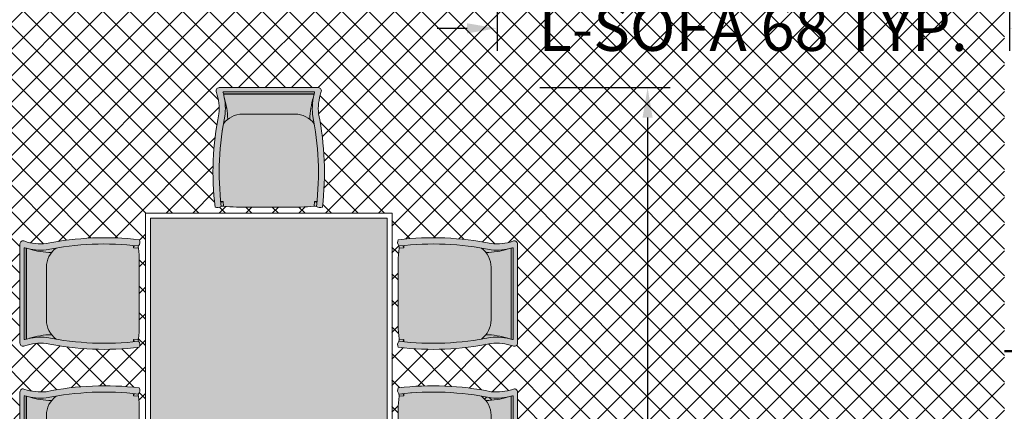
# Model space of a CAD drawing. Units: inches. Extents: x -466983 to 1020, y 324 to 318697.
# Tile 85 of 97: x 679 to 810, y 827 to 879. Entities that reach past the tile are written whole.
import ezdxf

# ---------------------------------------------------------------- set-up
doc = ezdxf.new("R2010")
doc.units = ezdxf.units.IN
doc.header["$MEASUREMENT"] = 0
for name, color, linetype, lineweight in [('A-ANNO-DIMS', 2, 'Continuous', 18), ('A-FLOR-PATT', 252, 'Continuous', 13), ('A-FURN', 8, 'Continuous', 18), ('A-WALL', 7, 'Continuous', 50)]:
    doc.layers.add(name, color=color, linetype=linetype, lineweight=lineweight)
doc.styles.get("Standard").update_dxf_attribs({"font": 'arial.ttf'})
doc.dimstyles.get("Standard").update_dxf_attribs({"dimtxt": 6, "dimasz": 4, "dimexe": 3, "dimexo": 3, "dimgap": 0.09, "dimtad": 0, "dimtih": 1, "dimtoh": 1, "dimdec": 1, "dimzin": 0, "dimdsep": 46, "dimlunit": 3, "dimtxsty": 'Standard', "dimcen": 0.09, "dimadec": 0, "dimazin": 0, "dimtfac": 1, "dimtdec": 1, "dimtofl": 0, "dimtmove": 0, "dimatfit": 3, "dimfxl": 1, "dimtolj": 1, "dimtzin": 0, "dimarcsym": 0})

# ---------------------------------------------------------------- blocks, each defined once
blk = doc.blocks.new('A$C51F1')
h = blk.add_hatch(color=256)
h.dxf.hatch_style = 1
h.paths.add_polyline_path([(0.4279, 0.4929), (0.026, 0.4929, 0.585109), (0.0153, 0.4737, -0.102523), (0.0249, 0.3863, 0.080461), (0.0093, 0.0091, 0.3023), (0.0338, 0.012, -0.012942), (0.0343, 0.0123, -0.080591), (0.05, 0.3835, 0.086627), (0.0435, 0.4661, -0.308377), (0.0433, 0.4665, -0.237278), (0.0433, 0.4671, 0.005839), (0.0418, 0.4726, -0.471786), (0.0436, 0.4758), (0.2273, 0.4758), (0.4111, 0.4758, -0.471786), (0.4129, 0.4726, 0.005839), (0.4114, 0.4671, -0.293853), (0.4112, 0.4664, 0.08699), (0.4047, 0.3835, -0.080655), (0.4203, 0.012, 0.301773), (0.4447, 0.0091, 0.080461), (0.4291, 0.3863, -0.102523), (0.4387, 0.4737, 0.587111)])
h.paths.add_polyline_path([(0.4107, 0.4676), (0.2273, 0.4676), (0.0439, 0.4676, 0.311255), (0.0433, 0.4671, -0.000568), (0.0434, 0.4666, -0.365297), (0.0439, 0.4668), (0.2273, 0.4668), (0.4107, 0.4668, -0.365297), (0.4113, 0.4666, -0.000568), (0.4114, 0.4671, 0.311255)], flags=17)
h = blk.add_hatch(color=256)
h.dxf.hatch_style = 1
h.paths.add_polyline_path([(0.4117, 0.3464, 0.23459), (0.3341, 0.3858), (0.2273, 0.3858), (0.1205, 0.3858, 0.165743), (0.061, 0.3649, 0.071703), (0.0463, 0.4542, -0.071168), (0.0502, 0.3861, 0.080361), (0.0343, 0.0123, -0.184513), (0.0429, 0.0127, 0.028193), (0.097, 0.0091), (0.227, 0.0091), (0.3571, 0.0091, 0.028193), (0.4111, 0.0127, -0.198751), (0.4203, 0.012, 0.072468)])
h.paths.add_polyline_path([(0.4084, 0.4542, -0.01323), (0.4113, 0.4666, 0.365297), (0.4107, 0.4668, 0.310553), (0.4107, 0.4676), (0.0439, 0.4676, 0.311255), (0.0433, 0.4671, -0.013798), (0.0463, 0.4542, -0.071703), (0.061, 0.3649, -0.165743), (0.1205, 0.3858), (0.2273, 0.3858), (0.3341, 0.3858, -0.165743), (0.3937, 0.3649, -0.071703)])
h.paths.add_polyline_path([(0.4047, 0.3835, -0.073923), (0.4084, 0.4542, 0.071703), (0.3937, 0.3649, -0.06627), (0.4117, 0.3464, 0.008137)], flags=17)
h.paths.add_polyline_path([(0.413, 0.473, 0.415817), (0.4111, 0.4758), (0.0436, 0.4758, 0.415817), (0.0416, 0.473, -0.006308), (0.0433, 0.4671, -0.311255), (0.0439, 0.4676), (0.4107, 0.4676, -0.336555), (0.4114, 0.4671, -0.006308)])
h = blk.add_hatch(color=256)
h.dxf.hatch_style = 1
h.paths.add_polyline_path([(0.4084, 0.4542, -0.01323), (0.4113, 0.4666, 0.365297), (0.4107, 0.4668), (0.2273, 0.4668), (0.0436, 0.4668, 0.193526), (0.0434, 0.4666, -0.01323), (0.0463, 0.4542, -0.071703), (0.061, 0.3649, -0.165743), (0.1205, 0.3858), (0.2273, 0.3858), (0.3341, 0.3858, -0.165743), (0.3937, 0.3649, -0.071703)])
at = {"color": 0}
for p, q in [((0.0436, 0.4758), (0.4111, 0.4758)), ((0.0439, 0.4676), (0.4107, 0.4676)), ((0.2273, 0.4668), (0.0439, 0.4668)), ((0.2273, 0.4668), (0.4107, 0.4668)), ((0.2273, 0.3858), (0.1205, 0.3858)), ((0.2273, 0.3858), (0.3341, 0.3858)), ((0.0417, 0.0321), (0.0321, 0.0321)), ((0.0417, 0.0321), (0.0326, 0.0278)), ((0.0435, 0.0127), (0.0417, 0.0321)), ((0.4112, 0.0127), (0.4129, 0.0321)), ((0.4129, 0.0321), (0.4225, 0.0321)), ((0.4129, 0.0321), (0.4221, 0.0278))]:
    blk.add_line(p, q, dxfattribs=at)
blk.add_lwpolyline([(0.4387, 0.4737, 0.102523), (0.4291, 0.3863, -0.080461), (0.4447, 0.0091, -0.3023), (0.4203, 0.012, 0.197932), (0.4111, 0.0127, -0.028193), (0.3571, 0.0091), (0.227, 0.0091), (0.097, 0.0091, -0.028193), (0.0429, 0.0127, 0.197932), (0.0338, 0.012, -0.3023), (0.0093, 0.0091, -0.080461), (0.0249, 0.3863, 0.102523), (0.0153, 0.4737, -0.587111), (0.0261, 0.4929), (0.4279, 0.4929, -0.587111)], format="xyb", close=True, dxfattribs=at)
for centre, radius, start, end in [((0.044, 0.4735), 0.00242, 100.345, 201.3742), ((-0.1898, 0.4063), 0.2409, 355.1793, 16.07), ((0.0439, 0.4669), 0.000725, 87.3762, 197.5208), ((0.0438, 0.4664), 0.000433, 71.7715, 189.2202), ((-0.2563, 0.3584), 0.3173, 1.1591, 17.5641), ((0.7109, 0.3584), 0.3173, 162.4359, 178.8409), ((0.6445, 0.4063), 0.2409, 164.0374, 185.4487), ((0.4107, 0.4669), 0.000725, 342.4792, 92.6238), ((0.4109, 0.4664), 0.000433, 350.7798, 108.2285), ((0.4106, 0.4735), 0.00242, 338.6258, 79.655), ((1.1976, 0.1501), 1.1714, 168.378, 186.769), ((0.1214, 0.2879), 0.0978, 90.5164, 143.1927), ((0.3332, 0.2879), 0.0978, 36.8073, 89.4836), ((-0.7314, 0.1497), 1.1599, 353.1854, 11.6291), ((0.0397, 0.0013), 0.012, 71.7536, 116.5375), ((0.4149, 0.0013), 0.012, 63.4625, 108.2464)]:
    blk.add_arc(centre, radius, start, end, dxfattribs=at)
blk = doc.blocks.new('Dining Table 1')
h = blk.add_hatch(color=256)
h.dxf.hatch_style = 1
h.set_gradient(color1=(0, 107, 0), color2=(254, 234, 185), name='INVSPHERICAL')
h.paths.add_polyline_path([(1939.98, 1142.68), (1908.44, 1142.68), (1908.44, 1061.84), (1939.98, 1061.84)])
at = {"ltscale": 0.5}
for points in [[(1907.78, 1143.33), (1907.78, 1061.19), (1940.64, 1061.19), (1940.64, 1143.33)], [(1908.44, 1142.68), (1908.44, 1061.84), (1939.98, 1061.84), (1939.98, 1142.68)]]:
    blk.add_lwpolyline(points, close=True, dxfattribs=at)
at = {"ltscale": 0.5, "xscale": 32.85880592291654, "yscale": 32.85880592291654, "zscale": 32.85880592291654}
blk.add_blockref('A$C51F1', (1916.75, 1143.86), dxfattribs=at)
at = {"ltscale": 0.5, "yscale": 32.85880592291654, "zscale": 32.85880592291654}
for p, xscale, rotation in [((1907.26, 1140.11), -32.85880592291654, 90), ((1941.16, 1140.11), 32.85880592291654, 270), ((1907.26, 1120.4), -32.85880592291654, 90), ((1941.16, 1120.4), 32.85880592291654, 270), ((1907.26, 1085.76), 32.85880592291654, 89.99999999999999), ((1941.16, 1085.76), -32.85880592291654, 270), ((1907.26, 1064.41), 32.85880592291654, 89.99999999999999), ((1941.16, 1064.41), -32.85880592291654, 270), ((1916.75, 1060.66), -32.85880592291654, 180)]:
    blk.add_blockref('A$C51F1', p, dxfattribs=dict(at, xscale=xscale, rotation=rotation))
blk = doc.blocks.new('*D71')
at = {"layer": 'A-ANNO-DIMS', "color": 0, "lineweight": -2, "transparency": 16777216}
for p, q in [((742.22, 885.15), (742.22, 874.91)), ((810.49, 885.15), (810.49, 874.91)), ((738.22, 877.91), (734.22, 877.91)), ((814.49, 877.91), (818.49, 877.91))]:
    blk.add_line(p, q, dxfattribs=at)
at = {"layer": 'A-ANNO-DIMS', "color": 0, "transparency": 16777216}
for points in [[(738.22, 878.58), (738.22, 877.24), (742.22, 877.91)], [(814.49, 878.58), (814.49, 877.24), (810.49, 877.91)]]:
    blk.add_solid(points, dxfattribs=at)
at = {"layer": 'Defpoints', "color": 0, "transparency": 16777216}
for p in [(742.22, 888.15), (810.49, 888.15), (742.22, 877.91)]:
    blk.add_point(p, dxfattribs=at)
at = {"layer": 'A-ANNO-DIMS', "color": 0, "transparency": 16777216, "insert": (776.35, 877.91), "char_height": 6, "attachment_point": 5}
blk.add_mtext('\\A1;L-SOFA 68 TYP.', dxfattribs=at)
blk = doc.blocks.new('*D111')
at = {"layer": 'A-ANNO-DIMS', "color": 0, "lineweight": -2, "transparency": 16777216}
for p, q in [((747.94, 870.02), (765.28, 870.02)), ((762.28, 866.02), (762.28, 815.42)), ((762.28, 758.43), (762.28, 809.03)), ((747.94, 754.43), (765.28, 754.43))]:
    blk.add_line(p, q, dxfattribs=at)
at = {"layer": 'A-ANNO-DIMS', "color": 0, "transparency": 16777216}
for points in [[(761.61, 866.02), (762.95, 866.02), (762.28, 870.02)], [(761.61, 758.43), (762.95, 758.43), (762.28, 754.43)]]:
    blk.add_solid(points, dxfattribs=at)
at = {"layer": 'Defpoints', "color": 0, "transparency": 16777216}
for p in [(744.94, 870.02), (762.28, 870.02), (744.94, 754.43)]:
    blk.add_point(p, dxfattribs=at)
at = {"layer": 'A-ANNO-DIMS', "color": 0, "transparency": 16777216, "insert": (762.28, 812.23), "char_height": 6, "attachment_point": 5}
blk.add_mtext('\\A1;DINING SET 116', dxfattribs=at)

msp = doc.modelspace()

# ---------------------------------------------------------------- hatches: boundary and pattern name
at = {"layer": 'A-FLOR-PATT', "transparency": 33554572}
h = msp.add_hatch(dxfattribs=at)
h.set_pattern_fill('ANSI37', color=256, scale=30)
h.set_pattern_definition([(45, (-1212.4137, -290.035), (-2.6516504, 2.6516504), []), (135, (-1212.4137, -290.035), (-2.6516504, -2.6516504), [])])
h.paths.add_polyline_path([(901.81, 1075.94), (900.61, 1075.94), (900.61, 1065.39), (899.39, 1065.39), (898.09, 1065.39), (892.84, 1058.71, -0.258377), (892.19, 1058.35), (879.98, 1058.35, -0.20177), (879.44, 1058.58), (874.08, 1065.39), (872.78, 1065.39), (871.56, 1065.39), (871.56, 1075.94), (813.81, 1075.94), (813.81, 1044.79), (832.39, 1044.79, -0.394795), (848.66, 1028.54), (848.66, 1009.94), (901.81, 1009.94), (901.81, 1015.94), (901.31, 1015.94), (871.31, 1015.94), (871.31, 1017.25), (871.33, 1017.25, -0.401453), (901.31, 1045.94), (901.81, 1045.94)])
edge = h.paths.add_edge_path(flags=16)
edge.add_line((847.77, 1068.95), (847.77, 1073.71))
edge.add_arc((849.23, 1073.71), 1.45, 90, 180, ccw=False)
edge.add_line((849.23, 1075.16), (864.49, 1075.16))
edge.add_arc((864.49, 1073.71), 1.45, 0, 90, ccw=False)
edge.add_line((865.95, 1073.71), (865.95, 1069))
edge.add_arc((832.64, 1068.98), 33.3, -20.6123, 0.0472, ccw=False)
edge.add_ellipse((856.86, 1058.48), major_axis=(0, 10.21), ratio=0.685919, start_angle=100.0088, end_angle=259.9912, ccw=False)
edge.add_arc((881.07, 1068.98), 33.3, 180.0472, 200.6123, ccw=False)
h.paths.add_polyline_path([(853.15, 1066.48), (853.15, 1066.45), (853.15, 1066.45, 0.433107), (852.92, 1066.68), (852.92, 1066.45), (853.15, 1066.45), (853.15, 1066.48), (853.09, 1066.61, 0.697939), (852.7, 1066.45), (852.7, 1066.45), (852.7, 1066.48), (852.92, 1067), (852.92, 1066.68, -0.396254)], flags=0)
h.paths.add_polyline_path([(861.02, 1066.48), (861.02, 1066.45), (861.02, 1066.45, 0.416404), (860.8, 1066.68), (860.8, 1066.45), (861.02, 1066.45), (861.02, 1066.48), (860.97, 1066.61, 0.713344), (860.57, 1066.45), (860.57, 1066.45), (860.57, 1066.48), (860.8, 1067), (860.8, 1066.68, -0.379973)], flags=0)
edge = h.paths.add_edge_path(flags=0)
edge.add_spline(control_points=[(861.13, 1065.79), (861.47, 1065.25), (861.61, 1065.02), (861.98, 1064.37), (862.19, 1063.94), (862.56, 1063.04), (862.72, 1062.56), (862.99, 1061.58), (863.09, 1061.07), (863.25, 1060.03), (863.29, 1059.5), (863.33, 1058.44), (863.32, 1057.91), (863.24, 1056.85), (863.17, 1056.33), (862.97, 1055.31), (862.84, 1054.81), (862.54, 1053.85), (862.36, 1053.39), (861.95, 1052.52), (861.73, 1052.12), (861.23, 1051.36), (860.97, 1051.02), (860.4, 1050.39), (860.11, 1050.12), (859.49, 1049.65), (859.18, 1049.45), (858.53, 1049.13), (858.2, 1049.01), (857.53, 1048.85), (857.2, 1048.81), (856.52, 1048.81), (856.19, 1048.85), (855.52, 1049.01), (855.19, 1049.13), (854.54, 1049.45), (854.23, 1049.64), (853.61, 1050.12), (853.32, 1050.39), (852.75, 1051.01), (852.49, 1051.36), (852, 1052.11), (851.77, 1052.52), (851.36, 1053.39), (851.18, 1053.85), (850.88, 1054.81), (850.75, 1055.31), (850.55, 1056.33), (850.48, 1056.85), (850.4, 1057.9), (850.39, 1058.44), (850.43, 1059.5), (850.47, 1060.03), (850.63, 1061.07), (850.73, 1061.58), (851, 1062.56), (851.16, 1063.04), (851.53, 1063.94), (851.73, 1064.37), (852.11, 1065.02), (852.25, 1065.25), (852.61, 1065.73)], knot_values=[3.915332, 3.915332, 3.915332, 3.915332, 4.013468, 4.013468, 4.175532, 4.175532, 4.337596, 4.337596, 4.49966, 4.49966, 4.661724, 4.661724, 4.823788, 4.823788, 4.985852, 4.985852, 5.147916, 5.147916, 5.30998, 5.30998, 5.472044, 5.472044, 5.634109, 5.634109, 5.796173, 5.796173, 5.958237, 5.958237, 6.120301, 6.120301, 6.282365, 6.282365, 6.444429, 6.444429, 6.606493, 6.606493, 6.768557, 6.768557, 6.930621, 6.930621, 7.092685, 7.092685, 7.254749, 7.254749, 7.416813, 7.416813, 7.578878, 7.578878, 7.740942, 7.740942, 7.903006, 7.903006, 8.06507, 8.06507, 8.227134, 8.227134, 8.389198, 8.389198, 8.551262, 8.551262, 8.65037, 8.65037, 8.65037, 8.65037], degree=3, periodic=0)
edge.add_line((852.64, 1065.79), (861.13, 1065.79))
edge = h.paths.add_edge_path(flags=0)
edge.add_ellipse((856.85, 1057.74), major_axis=(0, 7.79), ratio=0.687861, start_angle=0, end_angle=360)
h.paths.add_polyline_path([(848.86, 1069.39), (848.86, 1073.96, -0.414214), (849.95, 1075.05), (863.77, 1075.05, -0.414214), (864.86, 1073.96), (864.86, 1069.39, -0.388936), (864.52, 1069.03, -0.043561), (849.2, 1069.03, -0.388936)], flags=0)
h.paths.add_polyline_path([(853.1, 1068.11, -1), (852.68, 1068.11, -1)], flags=0)
edge = h.paths.add_edge_path(flags=0)
edge.add_ellipse((856.86, 1057.34), major_axis=(0, 2.21), ratio=0.657164, start_angle=0, end_angle=360)
h.paths.add_polyline_path([(861.04, 1068.11, -1), (860.62, 1068.11, -1)], flags=0)
edge = h.paths.add_edge_path()
edge.add_line((573.95, 1057.34), (573.95, 1075.94))
edge.add_line((573.95, 1075.94), (558.73, 1075.94))
edge.add_line((558.73, 1075.94), (558.73, 1065.39))
edge.add_line((558.73, 1065.39), (557.51, 1065.39))
edge.add_line((557.51, 1065.39), (556.21, 1065.39))
edge.add_line((556.21, 1065.39), (550.95, 1058.71))
edge.add_arc((550.3, 1059.12), 0.765, 270, 327.9483, ccw=False)
edge.add_line((550.3, 1058.35), (538.1, 1058.35))
edge.add_arc((538.1, 1059.12), 0.765, 224.3704, 270, ccw=False)
edge.add_line((537.55, 1058.58), (532.2, 1065.39))
edge.add_line((532.2, 1065.39), (530.9, 1065.39))
edge.add_line((530.9, 1065.39), (529.67, 1065.39))
edge.add_line((529.67, 1065.39), (529.67, 1075.94))
edge.add_line((529.67, 1075.94), (520.81, 1075.94))
edge.add_line((520.81, 1075.94), (520.81, 1045.94))
edge.add_line((520.81, 1045.94), (521.31, 1045.94))
edge.add_arc((521.31, 1015.94), 30, 2.5075, 90, ccw=False)
edge.add_line((551.28, 1017.25), (551.31, 1017.25))
edge.add_line((551.31, 1017.25), (551.31, 1015.94))
edge.add_line((551.31, 1015.94), (520.81, 1015.94))
edge.add_line((520.81, 1015.94), (520.81, 1009.94))
edge.add_line((520.81, 1009.94), (559.19, 1010.4))
edge.add_arc((559.19, 1011.86), 1.45, 180, 270, ccw=False)
edge.add_line((557.74, 1011.86), (557.74, 1016.56))
edge.add_arc((591.04, 1016.59), 33.3, 159.3877, 180.0472, ccw=False)
edge.add_ellipse((566.82, 1027.08), major_axis=(0, 10.21), ratio=0.685919, start_angle=280.0088, end_angle=439.9912, ccw=False)
edge.add_arc((542.61, 1016.59), 33.3, 0.0472, 20.6123, ccw=False)
edge.add_line((575.91, 1016.62), (575.91, 1011.86))
edge.add_arc((574.46, 1011.86), 1.45, -90, 0, ccw=False)
edge.add_line((574.46, 1010.4), (608.81, 1009.94))
edge.add_line((608.81, 1009.94), (608.81, 1041.09))
edge.add_line((608.81, 1041.09), (590.22, 1041.09))
edge.add_arc((590.78, 1057.91), 16.83, 181.9277, 268.1032, ccw=False)
edge = h.paths.add_edge_path()
edge.add_ellipse((494.24, 583.62), major_axis=(0, 10.21), ratio=0.685919, start_angle=280.0088, end_angle=439.9912, ccw=False)
edge.add_arc((470.03, 573.12), 33.3, 0.0472, 20.6123, ccw=False)
edge.add_line((503.33, 573.15), (503.33, 568.39))
edge.add_arc((501.88, 568.39), 1.45, -90, 0, ccw=False)
edge.add_line((501.88, 566.94), (539.81, 566.94))
edge.add_line((539.81, 566.94), (539.81, 572.94))
edge.add_line((539.81, 572.94), (539.31, 572.94))
edge.add_line((539.31, 572.94), (509.31, 572.94))
edge.add_line((509.31, 572.94), (509.31, 574.25))
edge.add_line((509.31, 574.25), (509.33, 574.25))
edge.add_arc((539.31, 572.94), 30, 90, 177.4925, ccw=False)
edge.add_line((539.31, 602.94), (539.81, 602.94))
edge.add_line((539.81, 602.94), (539.81, 626.94))
edge.add_line((539.81, 626.94), (531.77, 626.94))
edge.add_line((531.77, 626.94), (531.77, 616.39))
edge.add_line((531.77, 616.39), (530.55, 616.39))
edge.add_line((530.55, 616.39), (529.25, 616.39))
edge.add_line((529.25, 616.39), (523.71, 609.35))
edge.add_line((523.71, 609.35), (510.78, 609.35))
edge.add_line((510.78, 609.35), (505.24, 616.39))
edge.add_line((505.24, 616.39), (503.94, 616.39))
edge.add_line((503.94, 616.39), (502.72, 616.39))
edge.add_line((502.72, 616.39), (502.72, 626.94))
edge.add_line((502.72, 626.94), (481.7, 626.94))
edge.add_line((481.7, 626.94), (481.7, 611))
edge.add_arc((467.27, 611.47), 14.44, 271.9277, 358.1032, ccw=False)
edge.add_line((467.76, 597.05), (451.81, 597.05))
edge.add_line((451.81, 597.05), (451.81, 584.4))
edge.add_line((451.81, 584.4), (451.81, 566.94))
edge.add_line((451.81, 566.94), (486.61, 566.94))
edge.add_arc((486.61, 568.39), 1.45, 180, 270, ccw=False)
edge.add_line((485.16, 568.39), (485.16, 573.1))
edge.add_arc((518.46, 573.12), 33.3, 159.3877, 180.0472, ccw=False)
h.paths.add_polyline_path([(836.26, 1020.73), (879.89, 1020.73), (879.89, 1039.39), (836.26, 1039.39)], flags=25)
h.paths.add_polyline_path([(549.99, 1036.75), (593.61, 1036.75), (593.61, 1055.41), (549.99, 1055.41)], flags=24)
h.paths.add_polyline_path([(475.12, 595.6), (518.75, 595.6), (518.75, 614.25), (475.12, 614.25)], flags=24)
h = msp.add_hatch(dxfattribs=at)
h.set_pattern_fill('ANSI37', color=256, scale=20)
h.set_pattern_definition([(45, (-1212.4137, -290.035), (-1.767767, 1.767767), []), (135, (-1212.4137, -290.035), (-1.767767, -1.767767), [])])
h.paths.add_polyline_path([(809.81, 870.94), (809.81, 888.15), (807, 888.15), (802.66, 888.15), (789.38, 888.15), (786.28, 888.15, -0.414214), (785.5, 888.94), (785.5, 900.2), (785.5, 908.47, -0.414214), (786.81, 909.78, -0.414214), (785.5, 911.09), (785.5, 929.1, -0.414214), (786.81, 930.41, -0.414214), (785.5, 931.72), (785.5, 931.9, -0.414214), (784.19, 930.59), (766.72, 930.59, -0.412359), (765.41, 931.9, -0.413741), (764.11, 930.58), (744.58, 930.42, -0.416556), (743.79, 931.21), (743.79, 933.52), (742.22, 933.52), (742.22, 952.02, -0.001344), (743.79, 952.2), (743.79, 953.94), (678.59, 953.94), (678.59, 951.13), (678.59, 946.79), (678.59, 933.52), (678.59, 930.42, -0.414214), (677.81, 929.63), (666.55, 929.63), (658.27, 929.63, -0.414214), (656.96, 930.94, -0.414214), (655.66, 929.63), (637.64, 929.63, -0.414214), (636.33, 930.94, -0.414214), (635.02, 929.63), (634.84, 929.63, -0.414214), (636.15, 928.32), (636.15, 910.85, -0.412359), (634.85, 909.55, -0.413741), (636.17, 908.25), (636.32, 888.71, -0.416556), (635.54, 887.92), (633.23, 887.92), (633.23, 886.35), (614.72, 886.35, -0.001344), (614.54, 887.92), (612.81, 887.92), (612.81, 834.94), (612.81, 752.94), (612.81, 748.94), (612.81, 697.94), (654.81, 697.94), (654.81, 701.94), (715.81, 701.94), (715.81, 737.44), (774.29, 737.44), (774.29, 795.94), (809.81, 795.94)])
h.paths.add_polyline_path([(679.28, 849.58, 0.102523), (682.15, 849.26, -0.080461), (694.54, 849.77, -0.283899), (694.48, 849.01, 0.136605), (694.41, 848.81, -0.030441), (694.54, 846.89), (694.54, 842.62), (694.54, 838.35, -0.028219), (694.42, 836.57), (694.43, 836.57, 0.196187), (694.45, 836.27, -0.302897), (694.54, 835.47, -0.080461), (682.15, 835.98, 0.102523), (679.28, 835.66, -0.58611), (678.65, 836.02), (678.65, 849.22, -0.58611)], flags=16)
h.paths.add_polyline_path([(679.52, 848.65, 0.699597), (679.48, 848.63, 1.20716), (679.19, 848.74, 0.010621)], flags=0)
h.paths.add_polyline_path([(679.49, 836.56, -0.013798), (679.92, 836.66, -0.071703), (682.85, 837.14, -0.165743), (682.17, 839.1), (682.17, 842.61), (682.17, 846.06, -0.240616), (683.47, 848.68, -0.068263), (693.93, 849.01), (693.79, 848.71), (693.79, 849.02, 0.067332), (683.47, 848.68, 0.240616), (682.17, 846.06), (682.17, 842.61), (682.17, 839.1, 0.23459), (683.46, 836.55, 0.068093), (693.79, 836.2), (693.79, 836.51), (693.93, 836.21, -0.077215), (682.24, 836.78, 0.086627), (679.53, 836.57, -0.628402), (679.5, 836.57), (679.5, 836.61, 0.910458)], flags=0)
h.paths.add_polyline_path([(679.48, 848.64), (679.21, 848.65), (679.21, 836.57, 0.913566), (679.36, 836.59), (679.48, 836.58)], flags=0)
h.paths.add_polyline_path([(679.28, 829.86, 0.102523), (682.15, 829.55, -0.080461), (694.54, 830.06, -0.283899), (694.48, 829.29, 0.136605), (694.41, 829.1, -0.030441), (694.54, 827.18), (694.54, 822.9), (694.54, 818.63, -0.028219), (694.42, 816.85), (694.43, 816.85, 0.196187), (694.45, 816.56, -0.302897), (694.54, 815.75, -0.080461), (682.15, 816.26, 0.102523), (679.28, 815.95, -0.58611), (678.65, 816.3), (678.65, 829.51, -0.58611)], flags=16)
h.paths.add_polyline_path([(679.52, 828.94, 0.699597), (679.48, 828.92, 1.20716), (679.19, 829.03, 0.010621)], flags=0)
h.paths.add_polyline_path([(679.49, 816.85, -0.013798), (679.92, 816.94, -0.071703), (682.85, 817.43, -0.165743), (682.17, 819.39), (682.17, 822.89), (682.17, 826.34, -0.240616), (683.47, 828.96, -0.068263), (693.93, 829.29), (693.79, 828.99), (693.79, 829.31, 0.067332), (683.47, 828.96, 0.240616), (682.17, 826.34), (682.17, 822.89), (682.17, 819.39, 0.23459), (683.46, 816.84, 0.068093), (693.79, 816.48), (693.79, 816.8), (693.93, 816.49, -0.077215), (682.24, 817.07, 0.086627), (679.53, 816.85, -0.628402), (679.5, 816.86), (679.5, 816.89, 0.910458)], flags=0)
h.paths.add_polyline_path([(679.48, 828.92), (679.21, 828.93), (679.21, 816.86, 0.913566), (679.36, 816.87), (679.48, 816.87)], flags=0)
h.paths.add_polyline_path([(679.28, 810.15, 0.102523), (682.15, 809.83, -0.080461), (694.54, 810.34, -0.3023), (694.45, 809.54, 0.10023), (694.41, 809.39, -0.03057), (694.54, 807.46), (694.54, 803.19), (694.54, 798.92, -0.03057), (694.41, 796.99, 0.10023), (694.45, 796.84, -0.3023), (694.54, 796.04, -0.080461), (682.15, 796.55, 0.102523), (679.28, 796.23, -0.58611), (678.65, 796.59), (678.65, 809.79, -0.58611)], flags=16)
h.paths.add_polyline_path([(679.52, 809.24, 0.699597), (679.48, 809.22, 1.20716), (679.19, 809.33, 0.010621)], flags=0)
h.paths.add_polyline_path([(679.49, 797.15, -0.013798), (679.92, 797.25, -0.071703), (682.85, 797.73, -0.165743), (682.17, 799.69), (682.17, 803.2), (682.17, 806.65, -0.239349), (683.46, 809.26, -0.072465), (694.45, 809.54, 0.197932), (694.43, 809.24), (693.79, 809.3), (693.79, 809.61, 0.068093), (683.46, 809.26, 0.239349), (682.17, 806.65), (682.17, 803.2), (682.17, 799.69, 0.235854), (683.47, 797.13, 0.067332), (693.79, 796.79), (693.79, 797.1), (694.43, 797.16, 0.197932), (694.45, 796.86, -0.080419), (682.16, 797.38, 0.083867), (679.53, 797.16, -0.628402), (679.5, 797.16), (679.5, 797.2, 0.910458)], flags=0)
h.paths.add_polyline_path([(679.21, 809.24), (679.21, 797.16, 0.913566), (679.36, 797.18), (679.48, 797.17), (679.48, 809.23)], flags=0)
h.paths.add_polyline_path([(695.36, 853.3), (728.22, 853.3), (728.22, 771.15), (695.36, 771.15)], flags=16)
h.paths.add_polyline_path([(696.02, 852.64), (727.57, 852.64), (727.57, 771.81), (696.02, 771.81)], flags=0)
h.paths.add_polyline_path([(679.28, 788.79, 0.102523), (682.15, 788.47, -0.080461), (694.54, 788.98, -0.3023), (694.45, 788.18, 0.10023), (694.41, 788.03, -0.03057), (694.54, 786.1), (694.54, 781.83), (694.54, 777.56, -0.03057), (694.41, 775.63, 0.10023), (694.45, 775.48, -0.3023), (694.54, 774.68, -0.080461), (682.15, 775.19, 0.102523), (679.28, 774.88, -0.58611), (678.65, 775.23), (678.65, 788.43, -0.58611)], flags=16)
h.paths.add_polyline_path([(679.52, 787.88, 0.699597), (679.48, 787.87, 1.20716), (679.19, 787.97, 0.010621)], flags=0)
h.paths.add_polyline_path([(679.49, 775.79, -0.013798), (679.92, 775.89, -0.071703), (682.85, 776.38, -0.165743), (682.17, 778.33), (682.17, 781.84), (682.17, 785.29, -0.239349), (683.46, 787.9, -0.072465), (694.45, 788.18, 0.197932), (694.43, 787.88), (693.79, 787.94), (693.79, 788.26, 0.068093), (683.46, 787.9, 0.239349), (682.17, 785.29), (682.17, 781.84), (682.17, 778.33, 0.235854), (683.47, 775.77, 0.067332), (693.79, 775.43), (693.79, 775.74), (694.43, 775.8, 0.197932), (694.45, 775.5, -0.080419), (682.16, 776.02, 0.083867), (679.53, 775.8, -0.628402), (679.5, 775.81), (679.5, 775.84, 0.910458)], flags=0)
h.paths.add_polyline_path([(679.21, 787.88), (679.21, 775.8, 0.913566), (679.36, 775.82), (679.48, 775.81), (679.48, 787.87)], flags=0)
h.paths.add_polyline_path([(704.64, 854.12, -0.080461), (705.15, 866.52, 0.102523), (704.84, 869.39, -0.58611), (705.19, 870.02), (718.4, 870.02, -0.58611), (718.75, 869.39, 0.102523), (718.43, 866.52, -0.080461), (718.95, 854.12, -0.3023), (718.14, 854.22, 0.10023), (717.99, 854.26, -0.03057), (716.07, 854.12), (711.79, 854.12), (707.52, 854.12, -0.03057), (705.6, 854.26, 0.10023), (705.44, 854.22, -0.3023)], flags=16)
h.paths.add_polyline_path([(717.85, 869.15, 0.699597), (717.83, 869.19, 1.20716), (717.94, 869.47, 0.010621)], flags=0)
h.paths.add_polyline_path([(705.46, 854.22, -0.080419), (705.98, 866.51, 0.083867), (705.76, 869.13, -0.628402), (705.77, 869.16), (705.8, 869.16, 0.910458), (705.76, 869.17, -0.013798), (705.85, 868.75, -0.071703), (706.34, 865.81, -0.165743), (708.3, 866.5), (711.8, 866.5), (715.25, 866.5, -0.239349), (717.86, 865.2, -0.072465), (718.15, 854.22, 0.197932), (717.85, 854.24), (717.9, 854.88), (718.22, 854.88, 0.068093), (717.86, 865.2, 0.239349), (715.25, 866.5), (711.8, 866.5), (708.3, 866.5, 0.235854), (705.74, 865.19, 0.067332), (705.39, 854.88), (705.71, 854.88), (705.76, 854.24, 0.197932)], flags=16)
h.paths.add_polyline_path([(705.77, 869.46, 0.913566), (705.78, 869.3), (705.78, 869.19), (717.83, 869.19), (717.84, 869.46)], flags=0)
h.paths.add_polyline_path([(729.04, 842.62), (729.04, 846.89, -0.03057), (729.18, 848.82, 0.10023), (729.14, 848.97, -0.3023), (729.04, 849.77, -0.080461), (741.44, 849.26, 0.102523), (744.31, 849.58, -0.58611), (744.94, 849.22), (744.94, 836.02, -0.58611), (744.31, 835.66, 0.102523), (741.44, 835.98, -0.080461), (729.04, 835.47, -0.3023), (729.14, 836.27, 0.10023), (729.18, 836.42, -0.03057), (729.04, 838.35)], flags=16)
h.paths.add_polyline_path([(744.11, 836.58, 1.20716), (744.39, 836.48, 0.010621), (744.07, 836.57, 0.699597)], flags=0)
h.paths.add_polyline_path([(729.14, 836.27, 0.197932), (729.16, 836.57), (729.8, 836.51), (729.8, 836.2, 0.068093), (740.13, 836.55, 0.239349), (741.42, 839.16), (741.42, 842.61), (741.42, 846.12, 0.235854), (740.11, 848.68, 0.067332), (729.8, 849.02), (729.8, 848.71), (729.16, 848.65, 0.197932), (729.14, 848.95, -0.080419), (741.43, 848.43, 0.083867), (744.06, 848.65, -0.628402), (744.08, 848.65), (744.08, 848.61, 0.910458), (744.1, 848.66, -0.013798), (743.67, 848.56, -0.071703), (740.73, 848.08, -0.165743), (741.42, 846.12), (741.42, 842.61), (741.42, 839.16, -0.239349), (740.13, 836.55, -0.072465)], flags=0)
h.paths.add_polyline_path([(729.04, 830.06, -0.080461), (741.44, 829.55, 0.102523), (744.31, 829.86, -0.58611), (744.94, 829.51), (744.94, 816.3, -0.58611), (744.31, 815.95, 0.102523), (741.44, 816.26, -0.080461), (729.04, 815.75, -0.3023), (729.14, 816.55, 0.10023), (729.18, 816.71, -0.03057), (729.04, 818.63), (729.04, 822.9), (729.04, 827.18, -0.03057), (729.18, 829.1, 0.10023), (729.14, 829.25, -0.3023)], flags=16)
h.paths.add_polyline_path([(744.11, 816.87, 1.20716), (744.39, 816.76, 0.010621), (744.07, 816.85, 0.699597)], flags=0)
h.paths.add_polyline_path([(729.14, 829.24, -0.080419), (741.43, 828.71, 0.083867), (744.06, 828.93, -0.628402), (744.08, 828.93), (744.08, 828.9, 0.910458), (744.1, 828.94, -0.013798), (743.67, 828.84, -0.071703), (740.73, 828.36, -0.165743), (741.42, 826.4), (741.42, 822.89), (741.42, 819.44, -0.239349), (740.13, 816.84, -0.072465), (729.14, 816.55, 0.197932), (729.16, 816.85), (729.8, 816.8), (729.8, 816.48, 0.068093), (740.13, 816.84, 0.239349), (741.42, 819.44), (741.42, 822.89), (741.42, 826.4, 0.235854), (740.11, 828.96, 0.067332), (729.8, 829.31), (729.8, 828.99), (729.16, 828.94, 0.197932)], flags=16)
h.paths.add_polyline_path([(729.04, 810.34, -0.080461), (741.44, 809.83, 0.102523), (744.31, 810.15, -0.58611), (744.94, 809.79), (744.94, 796.59, -0.58611), (744.31, 796.23, 0.102523), (741.44, 796.55, -0.080461), (729.04, 796.04, -0.283899), (729.11, 796.8, 0.136605), (729.18, 797, -0.030441), (729.04, 798.92), (729.04, 803.19), (729.04, 807.46, -0.028219), (729.16, 809.24), (729.16, 809.24, 0.196187), (729.14, 809.54, -0.302897)], flags=16)
h.paths.add_polyline_path([(744.11, 797.17, 1.20716), (744.39, 797.07, 0.010621), (744.07, 797.16, 0.699597)], flags=0)
h.paths.add_polyline_path([(741.35, 809.03, 0.086627), (744.06, 809.24, -0.628402), (744.08, 809.24), (744.08, 809.2, 0.910458), (744.1, 809.25, -0.013798), (743.67, 809.15, -0.071703), (740.73, 808.67, -0.165743), (741.42, 806.71), (741.42, 803.2), (741.42, 799.75, -0.240616), (740.11, 797.13, -0.068263), (729.66, 796.8), (729.8, 797.1), (729.8, 796.79, 0.067332), (740.11, 797.13, 0.240616), (741.42, 799.75), (741.42, 803.2), (741.42, 806.71, 0.23459), (740.13, 809.26, 0.068093), (729.8, 809.61), (729.8, 809.3), (729.66, 809.6, -0.077215)], flags=0)
h.paths.add_polyline_path([(704.64, 770.33, -0.283899), (705.41, 770.27, 0.136605), (705.6, 770.19, -0.030441), (707.52, 770.33), (711.79, 770.33), (716.07, 770.33, -0.028219), (717.85, 770.21), (717.85, 770.21, 0.196187), (718.14, 770.23, -0.302897), (718.95, 770.33, -0.080461), (718.43, 757.94, 0.102523), (718.75, 755.06, -0.58611), (718.4, 754.43), (705.19, 754.43, -0.58611), (704.84, 755.06, 0.102523), (705.15, 757.94, -0.080461)], flags=16)
h.paths.add_polyline_path([(705.76, 755.3, 0.699597), (705.78, 755.26, 1.20716), (705.67, 754.98, 0.010621)], flags=0)
h.paths.add_polyline_path([(705.41, 769.72), (705.71, 769.58), (705.39, 769.58, 0.067332), (705.74, 759.26, 0.240616), (708.35, 757.95), (711.8, 757.95), (715.31, 757.95, 0.23459), (717.86, 759.25, 0.068093), (718.22, 769.58), (717.9, 769.58), (718.2, 769.72, -0.077215), (717.63, 758.03, 0.086627), (717.84, 755.32, -0.628402), (717.84, 755.29), (717.81, 755.29, 0.910458), (717.85, 755.28, -0.013798), (717.75, 755.71, -0.071703), (717.27, 758.64, -0.165743), (715.31, 757.95), (711.8, 757.95), (708.35, 757.95, -0.240616), (705.74, 759.26, -0.068263)], flags=0)
h.paths.add_polyline_path([(729.04, 788.98, -0.080461), (741.44, 788.47, 0.102523), (744.31, 788.79, -0.58611), (744.94, 788.43), (744.94, 775.23, -0.58611), (744.31, 774.88, 0.102523), (741.44, 775.19, -0.080461), (729.04, 774.68, -0.283899), (729.11, 775.44, 0.136605), (729.18, 775.64, -0.030441), (729.04, 777.56), (729.04, 781.83), (729.04, 786.1, -0.028219), (729.16, 787.88), (729.16, 787.88, 0.196187), (729.14, 788.18, -0.302897)], flags=16)
h.paths.add_polyline_path([(744.11, 775.82, 1.20716), (744.39, 775.71, 0.010621), (744.07, 775.8, 0.699597)], flags=0)
h.paths.add_polyline_path([(741.35, 787.67, 0.086627), (744.06, 787.88, -0.628402), (744.08, 787.88), (744.08, 787.84, 0.910458), (744.1, 787.89, -0.013798), (743.67, 787.79, -0.071703), (740.73, 787.31, -0.165743), (741.42, 785.35), (741.42, 781.84), (741.42, 778.39, -0.240616), (740.11, 775.77, -0.068263), (729.66, 775.44), (729.8, 775.74), (729.8, 775.43, 0.067332), (740.11, 775.77, 0.240616), (741.42, 778.39), (741.42, 781.84), (741.42, 785.35, 0.23459), (740.13, 787.9, 0.068093), (729.8, 788.26), (729.8, 787.94), (729.66, 788.24, -0.077215)], flags=0)
h.paths.add_polyline_path([(744.11, 848.64), (744.11, 836.58), (744.38, 836.57), (744.38, 848.65, 0.913566), (744.22, 848.63)], flags=0)
h.paths.add_polyline_path([(744.22, 828.92), (744.11, 828.92), (744.11, 816.87), (744.38, 816.86), (744.38, 828.93, 0.913566)], flags=0)
h.paths.add_polyline_path([(717.83, 755.26), (705.78, 755.26), (705.77, 754.99), (717.84, 754.99, 0.913566), (717.83, 755.15)], flags=0)
h.paths.add_polyline_path([(744.22, 809.22), (744.11, 809.23), (744.11, 797.17), (744.38, 797.16), (744.38, 809.24, 0.913566)], flags=0)
h.paths.add_polyline_path([(744.11, 787.87), (744.11, 775.81), (744.38, 775.8), (744.38, 787.88, 0.913566), (744.22, 787.86)], flags=0)
h.paths.add_polyline_path([(678.88, 877.12), (737.61, 877.12), (737.61, 899.51), (678.88, 899.51)], flags=24)

# ---------------------------------------------------------------- linework, layer by layer
at = {"layer": 'A-WALL'}
msp.add_line((813.81, 834.94), (809.81, 834.94), dxfattribs=at)

# ---------------------------------------------------------------- block references
at = {"layer": 'A-FURN'}
msp.add_blockref('Dining Table 1', (-1212.41, -290.04), dxfattribs=at)

# ---------------------------------------------------------------- dimensions: what is measured, and where the dimension line sits
at = {"layer": 'A-ANNO-DIMS'}
for base, p1, p2, angle, text, picture, middle in [((742.22, 877.91), (810.49, 888.15), (742.22, 888.15), 180, 'L-SOFA <> TYP.', '*D71', (776.35, 877.91)), ((762.28, 870.02), (744.94, 754.43), (744.94, 870.02), 90, 'DINING SET <>', '*D111', (762.28, 812.23))]:
    dim = msp.add_linear_dim(base=base, p1=p1, p2=p2, angle=angle, text=text, dimstyle='Standard', override={"dimdec": 0, "dimlfac": 1, "dimrnd": 0, "dimzin": 0, "dimdsep": 46, "dimlunit": 2}, dxfattribs=at)
    dim.commit()
    dim.dimension.update_dxf_attribs({"geometry": picture, "text_midpoint": middle})

doc.saveas('drawing.dxf')
